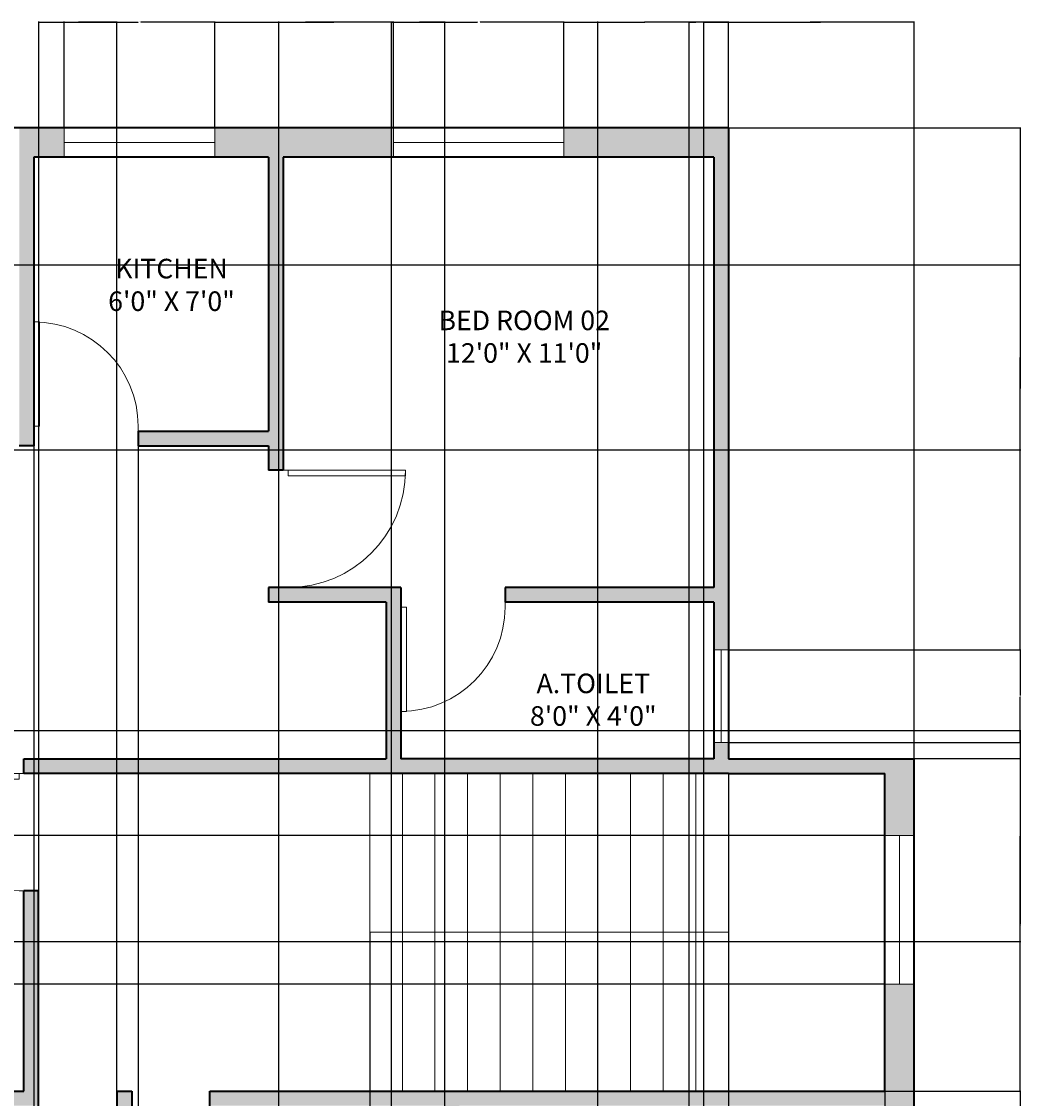
# Model space of a CAD drawing. Units: inches. Extents: x 2510 to 3056, y 673 to 1386.
# Tile 4 of 4: x 2749 to 3056, y 1056 to 1386. Entities that reach past the tile are written whole.
import ezdxf

# ---------------------------------------------------------------- set-up
doc = ezdxf.new("R2010")
doc.units = ezdxf.units.IN
for name, color, linetype, lineweight in [('A-ANNO-DIMS', 2, 'Continuous', 18), ('A-AREA-IDEN', 7, 'Continuous', 18), ('A-DOOR', 3, 'Continuous', 18), ('A-FLOR-STRS', 7, 'Continuous', 18), ('A-GLAZ', 4, 'Continuous', 18), ('A-WALL', 7, 'Continuous', 35), ('A-WALL-PATT', 252, 'Continuous', 13)]:
    doc.layers.add(name, color=color, linetype=linetype, lineweight=lineweight)
doc.styles.get("Standard").update_dxf_attribs({"font": 'arial.ttf'})
doc.dimstyles.get("Standard").update_dxf_attribs({"dimtxt": 0.18, "dimasz": 0.18, "dimexe": 0.18, "dimexo": 0.0625, "dimgap": 0.09, "dimtad": 0, "dimtih": 1, "dimtoh": 1, "dimdec": 4, "dimzin": 0, "dimdsep": 46, "dimtxsty": 'Standard', "dimcen": 0.09, "dimadec": 0, "dimazin": 0, "dimtfac": 1, "dimtdec": 4, "dimtofl": 0, "dimtmove": 0, "dimatfit": 3, "dimfxl": 1, "dimtolj": 1, "dimtzin": 0, "dimarcsym": 0})

# ---------------------------------------------------------------- blocks, each defined once
blk = doc.blocks.new('*U5')
for p, q in [((0, 0), (0, 6)), ((32, 0), (32, 6))]:
    blk.add_line(p, q)
blk.add_lwpolyline([(0, 0), (0, -32), (1.75, -32), (1.75, 0)], close=True)
blk.add_arc((0, 0), 32, 270, 0)
blk = doc.blocks.new('*U6')
for p, q in [((0, 0), (0, -6)), ((36, 0), (36, -6))]:
    blk.add_line(p, q)
blk.add_lwpolyline([(0, 0), (0, 36), (1.75, 36), (1.75, 0)], close=True)
blk.add_arc((0, 0), 36, 0, 90)
blk = doc.blocks.new('*U2')
for p, q in [((0, 0), (0, -6)), ((32, 0), (32, -6))]:
    blk.add_line(p, q)
blk.add_lwpolyline([(0, 0), (0, 32), (1.75, 32), (1.75, 0)], close=True)
blk.add_arc((0, 0), 32, 0, 90)
blk = doc.blocks.new('*U4')
for p, q in [((0, 0), (0, -6)), ((-36, 0), (-36, -6))]:
    blk.add_line(p, q)
blk.add_lwpolyline([(0, 0), (0, 36), (-1.75, 36), (-1.75, 0)], close=True)
blk.add_arc((0, 0), 36, 90, 180)
blk = doc.blocks.new('*U8')
for p, q in [((-24, 0), (-24, 6)), ((0, 0), (0, 6))]:
    blk.add_line(p, q)
blk.add_lwpolyline([(0, 0), (0, -24), (-1.75, -24), (-1.75, 0)], close=True)
blk.add_arc((0, 0), 24, 180, 270)
blk = doc.blocks.new('*U7')
for p, q in [((0, 0), (0, 6)), ((24, 0), (24, 6))]:
    blk.add_line(p, q)
blk.add_lwpolyline([(0, 0), (0, -24), (1.75, -24), (1.75, 0)], close=True)
blk.add_arc((0, 0), 24, 270, 0)
blk = doc.blocks.new('*D18')
at = {"layer": 'A-ANNO-DIMS', "color": 0, "lineweight": -2, "transparency": 16777216}
for p, q in [((2762.47, 1353.65), (2762.47, 1386.25)), ((2762.65, 1386.07), (2785.17, 1386.07)), ((2808.48, 1386.07), (2785.96, 1386.07)), ((2808.66, 1353.65), (2808.66, 1386.25))]:
    blk.add_line(p, q, dxfattribs=at)
at = {"layer": 'A-ANNO-DIMS', "color": 0, "transparency": 16777216}
for points in [[(2762.65, 1386.1), (2762.65, 1386.04), (2762.47, 1386.07)], [(2808.48, 1386.1), (2808.48, 1386.04), (2808.66, 1386.07)]]:
    blk.add_solid(points, dxfattribs=at)
at = {"layer": 'Defpoints', "color": 0, "transparency": 16777216}
for p in [(2808.66, 1386.07), (2762.47, 1353.59), (2808.66, 1353.59)]:
    blk.add_point(p, dxfattribs=at)
at = {"layer": 'A-ANNO-DIMS', "color": 0, "transparency": 16777216, "insert": (2785.57, 1386.07), "char_height": 0.18, "attachment_point": 5}
blk.add_mtext('\\A1;46.19', dxfattribs=at)
blk = doc.blocks.new('*D19')
at = {"layer": 'A-ANNO-DIMS', "color": 0, "lineweight": -2, "transparency": 16777216}
for p, q in [((2808.66, 1353.65), (2808.66, 1386.25)), ((2808.84, 1386.07), (2835.69, 1386.07)), ((2863.32, 1386.07), (2836.48, 1386.07)), ((2863.5, 1353.65), (2863.5, 1386.25))]:
    blk.add_line(p, q, dxfattribs=at)
at = {"layer": 'A-ANNO-DIMS', "color": 0, "transparency": 16777216}
for points in [[(2808.84, 1386.1), (2808.84, 1386.04), (2808.66, 1386.07)], [(2863.32, 1386.1), (2863.32, 1386.04), (2863.5, 1386.07)]]:
    blk.add_solid(points, dxfattribs=at)
at = {"layer": 'Defpoints', "color": 0, "transparency": 16777216}
for p in [(2863.5, 1386.07), (2808.66, 1353.59), (2863.5, 1353.59)]:
    blk.add_point(p, dxfattribs=at)
at = {"layer": 'A-ANNO-DIMS', "color": 0, "transparency": 16777216, "insert": (2836.08, 1386.07), "char_height": 0.18, "attachment_point": 5}
blk.add_mtext('\\A1;54.84', dxfattribs=at)
blk = doc.blocks.new('*D20')
at = {"layer": 'A-ANNO-DIMS', "color": 0, "lineweight": -2, "transparency": 16777216}
for p, q in [((2863.5, 1353.65), (2863.5, 1386.25)), ((2863.68, 1386.07), (2889.22, 1386.07)), ((2915.55, 1386.07), (2890.01, 1386.07)), ((2915.73, 1353.65), (2915.73, 1386.25))]:
    blk.add_line(p, q, dxfattribs=at)
at = {"layer": 'A-ANNO-DIMS', "color": 0, "transparency": 16777216}
for points in [[(2863.68, 1386.1), (2863.68, 1386.04), (2863.5, 1386.07)], [(2915.55, 1386.1), (2915.55, 1386.04), (2915.73, 1386.07)]]:
    blk.add_solid(points, dxfattribs=at)
at = {"layer": 'Defpoints', "color": 0, "transparency": 16777216}
for p in [(2915.73, 1386.07), (2863.5, 1353.59), (2915.73, 1353.59)]:
    blk.add_point(p, dxfattribs=at)
at = {"layer": 'A-ANNO-DIMS', "color": 0, "transparency": 16777216, "insert": (2889.61, 1386.07), "char_height": 0.18, "attachment_point": 5}
blk.add_mtext('\\A1;52.23', dxfattribs=at)
blk = doc.blocks.new('*D21')
at = {"layer": 'A-ANNO-DIMS', "color": 0, "lineweight": -2, "transparency": 16777216}
for p, q in [((2966.19, 1160.15), (2966.19, 1386.25)), ((2966.37, 1386.07), (2994.47, 1386.07)), ((3023.01, 1386.07), (2994.91, 1386.07)), ((3023.19, 1160.15), (3023.19, 1386.25))]:
    blk.add_line(p, q, dxfattribs=at)
at = {"layer": 'A-ANNO-DIMS', "color": 0, "transparency": 16777216}
for points in [[(2966.37, 1386.1), (2966.37, 1386.04), (2966.19, 1386.07)], [(3023.01, 1386.1), (3023.01, 1386.04), (3023.19, 1386.07)]]:
    blk.add_solid(points, dxfattribs=at)
at = {"layer": 'Defpoints', "color": 0, "transparency": 16777216}
for p in [(3023.19, 1386.07), (2966.19, 1160.09), (3023.19, 1160.09)]:
    blk.add_point(p, dxfattribs=at)
at = {"layer": 'A-ANNO-DIMS', "color": 0, "transparency": 16777216, "insert": (2994.69, 1386.07), "char_height": 0.18, "attachment_point": 5}
blk.add_mtext('\\A1;57', dxfattribs=at)
blk = doc.blocks.new('*D28')
at = {"layer": 'A-ANNO-DIMS', "color": 0, "lineweight": -2, "transparency": 16777216}
for p, q in [((3014.25, 1058.09), (3055.85, 1058.09)), ((3055.67, 1057.91), (3055.67, 1043.24)), ((3055.67, 1028.21), (3055.67, 1042.88)), ((3023.25, 1028.03), (3055.85, 1028.03))]:
    blk.add_line(p, q, dxfattribs=at)
at = {"layer": 'A-ANNO-DIMS', "color": 0, "transparency": 16777216}
for points in [[(3055.64, 1057.91), (3055.7, 1057.91), (3055.67, 1058.09)], [(3055.64, 1028.21), (3055.7, 1028.21), (3055.67, 1028.03)]]:
    blk.add_solid(points, dxfattribs=at)
at = {"layer": 'Defpoints', "color": 0, "transparency": 16777216}
for p in [(3014.19, 1058.09), (3055.67, 1058.09), (3023.19, 1028.03)]:
    blk.add_point(p, dxfattribs=at)
at = {"layer": 'A-ANNO-DIMS', "color": 0, "transparency": 16777216, "insert": (3055.67, 1043.06), "char_height": 0.18, "attachment_point": 5}
blk.add_mtext('\\A1;30.053', dxfattribs=at)
blk = doc.blocks.new('*D29')
at = {"layer": 'A-ANNO-DIMS', "color": 0, "lineweight": -2, "transparency": 16777216}
for p, q in [((3023.25, 1160.09), (3055.85, 1160.09)), ((3055.67, 1159.91), (3055.67, 1109.27)), ((3055.67, 1058.27), (3055.67, 1108.9)), ((3014.25, 1058.09), (3055.85, 1058.09))]:
    blk.add_line(p, q, dxfattribs=at)
at = {"layer": 'A-ANNO-DIMS', "color": 0, "transparency": 16777216}
for points in [[(3055.64, 1159.91), (3055.7, 1159.91), (3055.67, 1160.09)], [(3055.64, 1058.27), (3055.7, 1058.27), (3055.67, 1058.09)]]:
    blk.add_solid(points, dxfattribs=at)
at = {"layer": 'Defpoints', "color": 0, "transparency": 16777216}
for p in [(3023.19, 1160.09), (3055.67, 1160.09), (3014.19, 1058.09)]:
    blk.add_point(p, dxfattribs=at)
at = {"layer": 'A-ANNO-DIMS', "color": 0, "transparency": 16777216, "insert": (3055.67, 1109.09), "char_height": 0.18, "attachment_point": 5}
blk.add_mtext('\\A1;102', dxfattribs=at)
blk = doc.blocks.new('*D30')
at = {"layer": 'A-ANNO-DIMS', "color": 0, "lineweight": -2, "transparency": 16777216}
for p, q in [((2966.25, 1193.43), (3055.85, 1193.43)), ((3055.67, 1193.25), (3055.67, 1179.42)), ((3055.67, 1165.21), (3055.67, 1179.05)), ((2966.25, 1165.03), (3055.85, 1165.03))]:
    blk.add_line(p, q, dxfattribs=at)
at = {"layer": 'A-ANNO-DIMS', "color": 0, "transparency": 16777216}
for points in [[(3055.64, 1193.25), (3055.7, 1193.25), (3055.67, 1193.43)], [(3055.64, 1165.21), (3055.7, 1165.21), (3055.67, 1165.03)]]:
    blk.add_solid(points, dxfattribs=at)
at = {"layer": 'Defpoints', "color": 0, "transparency": 16777216}
for p in [(2966.19, 1193.43), (3055.67, 1193.43), (2966.19, 1165.03)]:
    blk.add_point(p, dxfattribs=at)
at = {"layer": 'A-ANNO-DIMS', "color": 0, "transparency": 16777216, "insert": (3055.67, 1179.23), "char_height": 0.18, "attachment_point": 5}
blk.add_mtext('\\A1;28.4', dxfattribs=at)
blk = doc.blocks.new('*D31')
at = {"layer": 'A-ANNO-DIMS', "color": 0, "lineweight": -2, "transparency": 16777216}
for p, q in [((2966.25, 1353.59), (3055.85, 1353.59)), ((3055.67, 1353.41), (3055.67, 1273.69)), ((3055.67, 1193.61), (3055.67, 1273.33)), ((2966.25, 1193.43), (3055.85, 1193.43))]:
    blk.add_line(p, q, dxfattribs=at)
at = {"layer": 'A-ANNO-DIMS', "color": 0, "transparency": 16777216}
for points in [[(3055.64, 1353.41), (3055.7, 1353.41), (3055.67, 1353.59)], [(3055.64, 1193.61), (3055.7, 1193.61), (3055.67, 1193.43)]]:
    blk.add_solid(points, dxfattribs=at)
at = {"layer": 'Defpoints', "color": 0, "transparency": 16777216}
for p in [(2966.19, 1353.59), (3055.67, 1353.59), (2966.19, 1193.43)]:
    blk.add_point(p, dxfattribs=at)
at = {"layer": 'A-ANNO-DIMS', "color": 0, "transparency": 16777216, "insert": (3055.67, 1273.51), "char_height": 0.18, "attachment_point": 5}
blk.add_mtext('\\A1;160.15', dxfattribs=at)
blk = doc.blocks.new('*D32')
at = {"layer": 'A-ANNO-DIMS', "color": 0, "lineweight": -2, "transparency": 16777216}
for p, q in [((3014.13, 1136.48), (2510.53, 1136.48)), ((2510.71, 1136.3), (2510.71, 1113.86)), ((2510.71, 1091.06), (2510.71, 1113.5)), ((3014.13, 1090.88), (2510.53, 1090.88))]:
    blk.add_line(p, q, dxfattribs=at)
at = {"layer": 'A-ANNO-DIMS', "color": 0, "transparency": 16777216}
for points in [[(2510.68, 1136.3), (2510.74, 1136.3), (2510.71, 1136.48)], [(2510.68, 1091.06), (2510.74, 1091.06), (2510.71, 1090.88)]]:
    blk.add_solid(points, dxfattribs=at)
at = {"layer": 'Defpoints', "color": 0, "transparency": 16777216}
for p in [(2510.71, 1136.48), (3014.19, 1136.48), (3014.19, 1090.88)]:
    blk.add_point(p, dxfattribs=at)
at = {"layer": 'A-ANNO-DIMS', "color": 0, "transparency": 16777216, "insert": (2510.71, 1113.68), "char_height": 0.18, "attachment_point": 5}
blk.add_mtext('\\A1;45.6', dxfattribs=at)
blk = doc.blocks.new('*D36')
at = {"layer": 'A-ANNO-DIMS', "color": 0, "lineweight": -2, "transparency": 16777216}
for p, q in [((2552.25, 1168.75), (3055.85, 1168.75)), ((3055.67, 1168.57), (3055.67, 1136.56)), ((3055.67, 1104.19), (3055.67, 1136.2)), ((2552.25, 1104.01), (3055.85, 1104.01))]:
    blk.add_line(p, q, dxfattribs=at)
at = {"layer": 'A-ANNO-DIMS', "color": 0, "transparency": 16777216}
for points in [[(3055.64, 1168.57), (3055.7, 1168.57), (3055.67, 1168.75)], [(3055.64, 1104.19), (3055.7, 1104.19), (3055.67, 1104.01)]]:
    blk.add_solid(points, dxfattribs=at)
at = {"layer": 'Defpoints', "color": 0, "transparency": 16777216}
for p in [(2552.19, 1168.75), (3055.67, 1168.75), (2552.19, 1104.01)]:
    blk.add_point(p, dxfattribs=at)
at = {"layer": 'A-ANNO-DIMS', "color": 0, "transparency": 16777216, "insert": (3055.67, 1136.38), "char_height": 0.18, "attachment_point": 5}
blk.add_mtext('\\A1;64.74', dxfattribs=at)
blk = doc.blocks.new('*D37')
at = {"layer": 'A-ANNO-DIMS', "color": 0, "lineweight": -2, "transparency": 16777216}
for p, q in [((2552.25, 1311.56), (3055.85, 1311.56)), ((3055.67, 1311.38), (3055.67, 1283.38)), ((3055.67, 1255.02), (3055.67, 1283.02)), ((2552.25, 1254.84), (3055.85, 1254.84))]:
    blk.add_line(p, q, dxfattribs=at)
at = {"layer": 'A-ANNO-DIMS', "color": 0, "transparency": 16777216}
for points in [[(3055.64, 1311.38), (3055.7, 1311.38), (3055.67, 1311.56)], [(3055.64, 1255.02), (3055.7, 1255.02), (3055.67, 1254.84)]]:
    blk.add_solid(points, dxfattribs=at)
at = {"layer": 'Defpoints', "color": 0, "transparency": 16777216}
for p in [(2552.19, 1311.56), (3055.67, 1311.56), (2552.19, 1254.84)]:
    blk.add_point(p, dxfattribs=at)
at = {"layer": 'A-ANNO-DIMS', "color": 0, "transparency": 16777216, "insert": (3055.67, 1283.2), "char_height": 0.18, "attachment_point": 5}
blk.add_mtext('\\A1;56.72', dxfattribs=at)
blk = doc.blocks.new('*D38')
at = {"layer": 'A-ANNO-DIMS', "color": 0, "lineweight": -2, "transparency": 16777216}
for p, q in [((2856.19, 1106.77), (2856.19, 672.93)), ((2966.19, 1106.77), (2966.19, 672.93)), ((2856.37, 673.11), (2910.91, 673.11)), ((2966.01, 673.11), (2911.47, 673.11))]:
    blk.add_line(p, q, dxfattribs=at)
at = {"layer": 'A-ANNO-DIMS', "color": 0, "transparency": 16777216}
for points in [[(2856.37, 673.14), (2856.37, 673.08), (2856.19, 673.11)], [(2966.01, 673.14), (2966.01, 673.08), (2966.19, 673.11)]]:
    blk.add_solid(points, dxfattribs=at)
at = {"layer": 'Defpoints', "color": 0, "transparency": 16777216}
for p in [(2856.19, 1106.84), (2966.19, 1106.84), (2966.19, 673.11)]:
    blk.add_point(p, dxfattribs=at)
at = {"layer": 'A-ANNO-DIMS', "color": 0, "transparency": 16777216, "insert": (2911.19, 673.11), "char_height": 0.18, "attachment_point": 5}
blk.add_mtext('\\A1;110', dxfattribs=at)
blk = doc.blocks.new('*D39')
at = {"layer": 'A-ANNO-DIMS', "color": 0, "lineweight": -2, "transparency": 16777216}
for p, q in [((2966.19, 1155.52), (2966.19, 672.93)), ((3014.19, 1155.52), (3014.19, 672.93)), ((2966.37, 673.11), (2989.97, 673.11)), ((3014.01, 673.11), (2990.42, 673.11))]:
    blk.add_line(p, q, dxfattribs=at)
at = {"layer": 'A-ANNO-DIMS', "color": 0, "transparency": 16777216}
for points in [[(2966.37, 673.14), (2966.37, 673.08), (2966.19, 673.11)], [(3014.01, 673.14), (3014.01, 673.08), (3014.19, 673.11)]]:
    blk.add_solid(points, dxfattribs=at)
at = {"layer": 'Defpoints', "color": 0, "transparency": 16777216}
for p in [(2966.19, 1155.59), (3014.19, 1155.59), (3014.19, 673.11)]:
    blk.add_point(p, dxfattribs=at)
at = {"layer": 'A-ANNO-DIMS', "color": 0, "transparency": 16777216, "insert": (2990.19, 673.11), "char_height": 0.18, "attachment_point": 5}
blk.add_mtext('\\A1;48', dxfattribs=at)
blk = doc.blocks.new('*D42')
at = {"layer": 'A-ANNO-DIMS', "color": 0, "lineweight": -2, "transparency": 16777216}
for p, q in [((2828.31, 719.15), (2828.31, 1386.25)), ((2828.49, 1386.07), (2845.18, 1386.07)), ((2862.66, 1386.07), (2845.97, 1386.07)), ((2862.84, 719.15), (2862.84, 1386.25))]:
    blk.add_line(p, q, dxfattribs=at)
at = {"layer": 'A-ANNO-DIMS', "color": 0, "transparency": 16777216}
for points in [[(2828.49, 1386.1), (2828.49, 1386.04), (2828.31, 1386.07)], [(2862.66, 1386.1), (2862.66, 1386.04), (2862.84, 1386.07)]]:
    blk.add_solid(points, dxfattribs=at)
at = {"layer": 'Defpoints', "color": 0, "transparency": 16777216}
for p in [(2862.84, 1386.07), (2828.31, 719.09), (2862.84, 719.09)]:
    blk.add_point(p, dxfattribs=at)
at = {"layer": 'A-ANNO-DIMS', "color": 0, "transparency": 16777216, "insert": (2845.57, 1386.07), "char_height": 0.18, "attachment_point": 5}
blk.add_mtext('\\A1;34.53', dxfattribs=at)
blk = doc.blocks.new('*D43')
at = {"layer": 'A-ANNO-DIMS', "color": 0, "lineweight": -2, "transparency": 16777216}
for p, q in [((2862.84, 719.15), (2862.84, 1386.25)), ((2863.02, 1386.07), (2870.56, 1386.07)), ((2879.01, 1386.07), (2871.47, 1386.07)), ((2879.19, 719.15), (2879.19, 1386.25))]:
    blk.add_line(p, q, dxfattribs=at)
at = {"layer": 'A-ANNO-DIMS', "color": 0, "transparency": 16777216}
for points in [[(2863.02, 1386.1), (2863.02, 1386.04), (2862.84, 1386.07)], [(2879.01, 1386.1), (2879.01, 1386.04), (2879.19, 1386.07)]]:
    blk.add_solid(points, dxfattribs=at)
at = {"layer": 'Defpoints', "color": 0, "transparency": 16777216}
for p in [(2879.19, 1386.07), (2862.84, 719.09), (2879.19, 719.09)]:
    blk.add_point(p, dxfattribs=at)
at = {"layer": 'A-ANNO-DIMS', "color": 0, "transparency": 16777216, "insert": (2871.02, 1386.07), "char_height": 0.18, "attachment_point": 5}
blk.add_mtext('\\A1;16.354', dxfattribs=at)
blk = doc.blocks.new('*D44')
at = {"layer": 'A-ANNO-DIMS', "color": 0, "lineweight": -2, "transparency": 16777216}
for p, q in [((2754.69, 1058.15), (2754.69, 1386.25)), ((2754.87, 1386.07), (2766.47, 1386.07)), ((2778.51, 1386.07), (2766.91, 1386.07)), ((2778.69, 1058.15), (2778.69, 1386.25))]:
    blk.add_line(p, q, dxfattribs=at)
at = {"layer": 'A-ANNO-DIMS', "color": 0, "transparency": 16777216}
for points in [[(2754.87, 1386.1), (2754.87, 1386.04), (2754.69, 1386.07)], [(2778.51, 1386.1), (2778.51, 1386.04), (2778.69, 1386.07)]]:
    blk.add_solid(points, dxfattribs=at)
at = {"layer": 'Defpoints', "color": 0, "transparency": 16777216}
for p in [(2778.69, 1386.07), (2754.69, 1058.09), (2778.69, 1058.09)]:
    blk.add_point(p, dxfattribs=at)
at = {"layer": 'A-ANNO-DIMS', "color": 0, "transparency": 16777216, "insert": (2766.69, 1386.07), "char_height": 0.18, "attachment_point": 5}
blk.add_mtext('\\A1;24', dxfattribs=at)
blk = doc.blocks.new('*D46')
at = {"layer": 'A-ANNO-DIMS', "color": 0, "lineweight": -2, "transparency": 16777216}
for p, q in [((2753.19, 1256.02), (2753.19, 672.93)), ((2785.19, 1256.02), (2785.19, 672.93)), ((2753.37, 673.11), (2768.97, 673.11)), ((2785.01, 673.11), (2769.41, 673.11))]:
    blk.add_line(p, q, dxfattribs=at)
at = {"layer": 'A-ANNO-DIMS', "color": 0, "transparency": 16777216}
for points in [[(2753.37, 673.14), (2753.37, 673.08), (2753.19, 673.11)], [(2785.01, 673.14), (2785.01, 673.08), (2785.19, 673.11)]]:
    blk.add_solid(points, dxfattribs=at)
at = {"layer": 'Defpoints', "color": 0, "transparency": 16777216}
for p in [(2753.19, 1256.09), (2785.19, 1256.09), (2785.19, 673.11)]:
    blk.add_point(p, dxfattribs=at)
at = {"layer": 'A-ANNO-DIMS', "color": 0, "transparency": 16777216, "insert": (2769.19, 673.11), "char_height": 0.18, "attachment_point": 5}
blk.add_mtext('\\A1;32', dxfattribs=at)
blk = doc.blocks.new('*D47')
at = {"layer": 'A-ANNO-DIMS', "color": 0, "lineweight": -2, "transparency": 16777216}
for p, q in [((2926.19, 750.65), (2926.19, 1386.25)), ((2926.37, 1386.07), (2939.97, 1386.07)), ((2954.01, 1386.07), (2940.41, 1386.07)), ((2954.19, 750.65), (2954.19, 1386.25))]:
    blk.add_line(p, q, dxfattribs=at)
at = {"layer": 'A-ANNO-DIMS', "color": 0, "transparency": 16777216}
for points in [[(2926.37, 1386.1), (2926.37, 1386.04), (2926.19, 1386.07)], [(2954.01, 1386.1), (2954.01, 1386.04), (2954.19, 1386.07)]]:
    blk.add_solid(points, dxfattribs=at)
at = {"layer": 'Defpoints', "color": 0, "transparency": 16777216}
for p in [(2954.19, 1386.07), (2926.19, 750.59), (2954.19, 750.59)]:
    blk.add_point(p, dxfattribs=at)
at = {"layer": 'A-ANNO-DIMS', "color": 0, "transparency": 16777216, "insert": (2940.19, 1386.07), "char_height": 0.18, "attachment_point": 5}
blk.add_mtext('\\A1;28', dxfattribs=at)
blk = doc.blocks.new('*D56')
at = {"layer": 'A-ANNO-DIMS', "color": 0, "lineweight": -2, "transparency": 16777216}
for p, q in [((2954.19, 750.65), (2954.19, 1386.25)), ((2954.37, 1386.07), (2956.18, 1386.07)), ((2958.51, 1386.07), (2956.7, 1386.07)), ((2958.69, 750.65), (2958.69, 1386.25))]:
    blk.add_line(p, q, dxfattribs=at)
at = {"layer": 'A-ANNO-DIMS', "color": 0, "transparency": 16777216}
for points in [[(2954.37, 1386.1), (2954.37, 1386.04), (2954.19, 1386.07)], [(2958.51, 1386.1), (2958.51, 1386.04), (2958.69, 1386.07)]]:
    blk.add_solid(points, dxfattribs=at)
at = {"layer": 'Defpoints', "color": 0, "transparency": 16777216}
for p in [(2958.69, 1386.07), (2954.19, 750.59), (2958.69, 750.59)]:
    blk.add_point(p, dxfattribs=at)
at = {"layer": 'A-ANNO-DIMS', "color": 0, "transparency": 16777216, "insert": (2956.44, 1386.07), "char_height": 0.18, "attachment_point": 5}
blk.add_mtext('\\A1;4.5', dxfattribs=at)
blk = doc.blocks.new('*D58')
at = {"layer": 'A-ANNO-DIMS', "color": 0, "lineweight": -2, "transparency": 16777216}
for p, q in [((2958.69, 705.65), (2958.69, 1386.25)), ((2958.87, 1386.07), (2990.62, 1386.07)), ((3023.01, 1386.07), (2991.27, 1386.07)), ((3023.19, 705.65), (3023.19, 1386.25))]:
    blk.add_line(p, q, dxfattribs=at)
at = {"layer": 'A-ANNO-DIMS', "color": 0, "transparency": 16777216}
for points in [[(2958.87, 1386.1), (2958.87, 1386.04), (2958.69, 1386.07)], [(3023.01, 1386.1), (3023.01, 1386.04), (3023.19, 1386.07)]]:
    blk.add_solid(points, dxfattribs=at)
at = {"layer": 'Defpoints', "color": 0, "transparency": 16777216}
for p in [(3023.19, 1386.07), (2958.69, 705.59), (3023.19, 705.59)]:
    blk.add_point(p, dxfattribs=at)
at = {"layer": 'A-ANNO-DIMS', "color": 0, "transparency": 16777216, "insert": (2990.94, 1386.07), "char_height": 0.18, "attachment_point": 5}
blk.add_mtext('\\A1;64.5', dxfattribs=at)
blk = doc.blocks.new('*D59')
at = {"layer": 'A-ANNO-DIMS', "color": 0, "lineweight": -2, "transparency": 16777216}
for p, q in [((2915.73, 1353.65), (2915.73, 1386.25)), ((2915.91, 1386.07), (2940.57, 1386.07)), ((2966.01, 1386.07), (2941.35, 1386.07)), ((2966.19, 1353.65), (2966.19, 1386.25))]:
    blk.add_line(p, q, dxfattribs=at)
at = {"layer": 'A-ANNO-DIMS', "color": 0, "transparency": 16777216}
for points in [[(2915.91, 1386.1), (2915.91, 1386.04), (2915.73, 1386.07)], [(2966.01, 1386.1), (2966.01, 1386.04), (2966.19, 1386.07)]]:
    blk.add_solid(points, dxfattribs=at)
at = {"layer": 'Defpoints', "color": 0, "transparency": 16777216}
for p in [(2966.19, 1386.07), (2915.73, 1353.59), (2966.19, 1353.59)]:
    blk.add_point(p, dxfattribs=at)
at = {"layer": 'A-ANNO-DIMS', "color": 0, "transparency": 16777216, "insert": (2940.96, 1386.07), "char_height": 0.18, "attachment_point": 5}
blk.add_mtext('\\A1;50.46', dxfattribs=at)

msp = doc.modelspace()

# ---------------------------------------------------------------- hatches: boundary and pattern name
at = {"layer": 'A-WALL-PATT'}
h = msp.add_hatch(color=256, dxfattribs=at)
h.dxf.hatch_style = 1
h.paths.add_polyline_path([(2580.5162, 1353.5862), (2543.1924, 1353.5862), (2543.1924, 1311.5591), (2552.1924, 1311.5591), (2552.1924, 1344.5862), (2580.5162, 1344.5862)])
h.paths.add_polyline_path([(2720.7125, 1353.5862), (2648.0497, 1353.5862), (2648.0497, 1344.5862), (2696.1924, 1344.5862), (2696.1924, 1208.0862), (2700.6924, 1208.0862), (2700.6924, 1256.0862), (2716.6924, 1256.0862), (2716.6924, 1260.5862), (2700.6924, 1260.5862), (2700.6924, 1344.5862), (2720.7125, 1344.5862)])
h.paths.add_polyline_path([(2762.4727, 1353.5862), (2748.6924, 1353.5862), (2748.6924, 1344.5862), (2748.6924, 1256.0862), (2753.1924, 1256.0862), (2753.1924, 1262.0862), (2753.1924, 1294.0862), (2753.1924, 1344.5862), (2762.4727, 1344.5862)])
h.paths.add_polyline_path([(2863.5016, 1353.5862), (2808.6621, 1353.5862), (2808.6621, 1344.5862), (2825.1924, 1344.5862), (2825.1924, 1260.5862), (2785.1924, 1260.5862), (2785.1924, 1256.0862), (2825.1924, 1256.0862), (2825.1924, 1248.5862), (2829.6924, 1248.5862), (2829.6924, 1344.5862), (2863.5016, 1344.5862)])
h.paths.add_polyline_path([(2966.1924, 1353.5862), (2915.7284, 1353.5862), (2915.7284, 1344.5862), (2961.6924, 1344.5862), (2961.6924, 1212.5862), (2897.6924, 1212.5862), (2897.6924, 1208.0862), (2961.6924, 1208.0862), (2961.6924, 1193.4346), (2966.1924, 1193.4346), (2966.1924, 1208.0862)])
h.paths.add_polyline_path([(2660.1924, 1212.5862), (2552.1924, 1212.5862), (2552.1924, 1254.8401), (2543.1924, 1254.8401), (2543.1924, 1168.7504), (2552.1924, 1168.7504), (2552.1924, 1208.0862), (2660.1924, 1208.0862)])
h.paths.add_polyline_path([(3023.1924, 1160.0862), (2966.1924, 1160.0862), (2966.1924, 1165.033), (2961.6924, 1165.033), (2961.6924, 1160.0862), (2865.6924, 1160.0862), (2865.6924, 1212.5862), (2825.1924, 1212.5862), (2825.1924, 1208.0862), (2861.1924, 1208.0862), (2861.1924, 1160.0862), (2750.1527, 1160.0862), (2750.1527, 1155.5862), (2754.6527, 1155.5862), (2966.1924, 1155.5862), (3014.1924, 1155.5862), (3014.1924, 1136.4806), (3023.1924, 1136.4806)])
h.paths.add_polyline_path([(3023.1924, 1090.8839), (3014.1924, 1090.8839), (3014.1924, 1058.0862), (2807.1924, 1058.0862), (2807.1924, 1053.5862), (2879.1924, 1053.5862), (2879.1924, 929.0862), (2883.6924, 929.0862), (2883.6924, 935.0862), (2883.6924, 971.0862), (2883.6924, 1053.5862), (3014.1924, 1053.5862), (3014.1924, 1028.0329), (3023.1924, 1028.0329)])
h.paths.add_polyline_path([(3023.1924, 970.6943), (3014.1924, 970.6943), (3014.1924, 933.5862), (2919.6924, 933.5862), (2919.6924, 929.0862), (2927.1924, 929.0862), (2927.1924, 907.0862), (2931.6924, 907.0862), (2931.6924, 929.0862), (3014.1924, 929.0862), (3014.1924, 918.5377), (3023.1924, 918.5377)])
h.paths.add_polyline_path([(3023.1924, 886.219), (3014.1924, 886.219), (3014.1924, 875.0862), (2927.1924, 875.0862), (2879.1924, 875.0862), (2879.1924, 870.5862), (2885.1924, 870.5862), (2921.1924, 870.5862), (3014.1924, 870.5862), (3014.1924, 835.4806), (3023.1924, 835.4806)])
h.paths.add_polyline_path([(3023.1924, 775.6299), (3014.1924, 775.6299), (3014.1924, 746.0862), (3023.1924, 746.0862)])
h.paths.add_polyline_path([(2958.6924, 750.5862), (2954.1924, 750.5862), (2954.1924, 744.5862), (2954.1924, 716.5862), (2954.1924, 710.0862), (2910.6841, 710.0862), (2910.6841, 705.5862), (2958.6924, 705.5862)])
h.paths.add_polyline_path([(2926.1924, 750.5862), (2883.6924, 750.5862), (2883.6924, 834.5862), (2879.1924, 834.5862), (2879.1924, 819.5862), (2815.1924, 819.5862), (2815.1924, 815.0862), (2879.1924, 815.0862), (2879.1924, 746.0862), (2879.1924, 719.0862), (2862.8388, 719.0862), (2862.8388, 714.5862), (2879.1924, 714.5862), (2879.1924, 705.5862), (2883.6924, 705.5862), (2883.6924, 710.0862), (2883.6924, 746.0862), (2926.1924, 746.1758)])
h.paths.add_polyline_path([(2682.6924, 815.0862), (2746.6924, 815.0862), (2746.6924, 819.5862), (2682.6924, 819.5862), (2682.6924, 834.5862), (2678.1924, 834.5862), (2678.1924, 750.5862), (2639.6924, 750.5862), (2639.6924, 746.0862), (2678.1924, 746.0862), (2678.1924, 710.0862), (2678.1924, 705.5862), (2682.6924, 705.5862), (2682.6924, 714.5862), (2699.7376, 714.5862), (2699.7376, 719.0862), (2682.6924, 719.0862), (2682.6924, 746.0862)])
h.paths.add_polyline_path([(2650.2761, 710.0862), (2607.6924, 710.0862), (2607.6924, 750.5862), (2603.1924, 750.5862), (2603.1924, 705.5862), (2607.6924, 705.5862), (2650.2761, 705.5862)])
h.paths.add_polyline_path([(2552.1924, 777.7158), (2543.1924, 777.7158), (2543.1924, 746.0862), (2552.1924, 746.0862)])
h.paths.add_polyline_path([(2828.3093, 719.0862), (2783.1924, 719.0862), (2783.1924, 815.0862), (2783.1924, 1058.0862), (2778.6924, 1058.0862), (2778.6924, 815.0862), (2778.6924, 719.0862), (2743.8813, 719.0862), (2743.8813, 714.5862), (2778.6924, 714.5862), (2828.3093, 714.5862)])
h.paths.add_polyline_path([(2642.1924, 933.5862), (2552.1924, 933.5862), (2552.1924, 965.3494), (2543.1924, 965.3494), (2543.1924, 907.809), (2552.1924, 907.809), (2552.1924, 929.0862), (2630.1924, 929.0862), (2630.1924, 907.0862), (2634.6924, 907.0862), (2634.6924, 929.0862), (2642.1924, 929.0862)])
h.paths.add_polyline_path([(2682.6924, 875.0862), (2552.1924, 875.0862), (2543.1924, 875.0862), (2543.1924, 832.3664), (2552.1924, 832.3664), (2552.1924, 870.5862), (2634.6924, 870.5862), (2682.6924, 870.5862)])
h.paths.add_polyline_path([(2754.6527, 1119.5862), (2750.1527, 1119.5862), (2750.1527, 1058.0862), (2552.1924, 1058.0862), (2552.1924, 1104.0128), (2543.1924, 1104.0128), (2543.1924, 1017.3235), (2552.1924, 1017.3235), (2552.1924, 1053.5862), (2678.1924, 1053.5862), (2678.1924, 929.0862), (2682.6924, 929.0862), (2682.6924, 1053.5862), (2754.6527, 1053.5862)])

# ---------------------------------------------------------------- linework, layer by layer
at = {"layer": 'A-FLOR-STRS'}
for p, q in [((2856.1924, 1155.5862), (2856.1924, 1058.0862)), ((2866.1924, 1155.5862), (2866.1924, 1058.0862)), ((2876.1924, 1155.5862), (2876.1924, 1058.0862)), ((2886.1924, 1155.5862), (2886.1924, 1058.0862)), ((2896.1924, 1155.5862), (2896.1924, 1058.0862)), ((2906.1924, 1155.5862), (2906.1924, 1058.0862)), ((2916.1924, 1155.5862), (2916.1924, 1058.0862)), ((2926.1924, 1155.5862), (2926.1924, 1058.0862)), ((2936.1924, 1155.5862), (2936.1924, 1058.0862)), ((2946.1924, 1155.5862), (2946.1924, 1058.0862)), ((2956.1924, 1155.5862), (2956.1924, 1058.0862)), ((2966.1924, 1155.5862), (2966.1924, 1058.0862)), ((2966.1924, 1106.8362), (2856.1924, 1106.8362))]:
    msp.add_line(p, q, dxfattribs=at)
at = {"layer": 'A-GLAZ'}
for p, q in [((2762.4727, 1344.5862), (2762.4727, 1353.5862)), ((2808.6621, 1344.5862), (2808.6621, 1353.5862)), ((2863.5016, 1344.5862), (2863.5016, 1353.5862)), ((2915.7284, 1353.5862), (2915.7284, 1344.5862)), ((2762.4727, 1349.0862), (2808.6621, 1349.0862)), ((2863.5016, 1349.0862), (2915.7284, 1349.0862)), ((2961.6924, 1193.4346), (2966.1924, 1193.4346)), ((2963.9424, 1165.033), (2963.9424, 1193.4346)), ((2961.6924, 1165.033), (2966.1924, 1165.033)), ((3014.1924, 1136.4806), (3023.1924, 1136.4806)), ((3018.6924, 1090.8839), (3018.6924, 1136.4806)), ((3014.1924, 1090.8839), (3023.1924, 1090.8839))]:
    msp.add_line(p, q, dxfattribs=at)
at = {"layer": 'A-WALL'}
for p, q in [((2966.1924, 1353.5862), (2543.1924, 1353.5862)), ((2966.1924, 1353.5862), (2966.1924, 1208.0862)), ((2753.1924, 1344.5862), (2753.1924, 1256.0862)), ((2825.1924, 1344.5862), (2753.1924, 1344.5862)), ((2825.1924, 1344.5862), (2825.1924, 1260.5862)), ((2961.6924, 1344.5862), (2829.6924, 1344.5862)), ((2829.6924, 1344.5862), (2829.6924, 1248.5862)), ((2961.6924, 1344.5862), (2961.6924, 1212.5862)), ((2785.1924, 1260.5862), (2785.1924, 1256.0862)), ((2785.1924, 1260.5862), (2825.1924, 1260.5862)), ((2753.1924, 1256.0862), (2748.6924, 1256.0862)), ((2785.1924, 1256.0862), (2825.1924, 1256.0862)), ((2825.1924, 1256.0862), (2825.1924, 1248.5862)), ((2829.6924, 1248.5862), (2825.1924, 1248.5862)), ((2825.1924, 1212.5862), (2825.1924, 1208.0862)), ((2865.6924, 1212.5862), (2825.1924, 1212.5862)), ((2865.6924, 1212.5862), (2865.6924, 1160.0862)), ((2961.6924, 1212.5862), (2897.6924, 1212.5862)), ((2897.6924, 1212.5862), (2897.6924, 1208.0862)), ((2861.1924, 1208.0862), (2825.1924, 1208.0862)), ((2861.1924, 1208.0862), (2861.1924, 1160.0862)), ((2961.6924, 1208.0862), (2897.6924, 1208.0862)), ((2961.6924, 1208.0862), (2961.6924, 1160.0862)), ((2966.1924, 1208.0862), (2966.1924, 1160.0862)), ((2750.1527, 1160.0862), (2861.1924, 1160.0862)), ((2750.1527, 1155.5862), (2750.1527, 1160.0862)), ((2961.6924, 1160.0862), (2865.6924, 1160.0862)), ((2966.1924, 1160.0862), (3023.1924, 1160.0862)), ((3023.1924, 705.5862), (3023.1924, 1160.0862)), ((2966.1924, 1155.5862), (2750.1527, 1155.5862)), ((2966.1924, 1155.5862), (3014.1924, 1155.5862)), ((3014.1924, 1058.0862), (3014.1924, 1155.5862)), ((2750.1527, 1058.0862), (2750.1527, 1119.5862)), ((2754.6527, 1119.5862), (2750.1527, 1119.5862)), ((2754.6527, 1053.5862), (2754.6527, 1119.5862)), ((2552.1924, 1058.0862), (2750.1527, 1058.0862)), ((2778.6924, 1058.0862), (2778.6924, 815.0862)), ((2778.6924, 1058.0862), (2783.1924, 1058.0862)), ((2783.1924, 1058.0862), (2783.1924, 815.0862)), ((2807.1924, 1053.5862), (2807.1924, 1058.0862)), ((2807.1924, 1058.0862), (3014.1924, 1058.0862))]:
    msp.add_line(p, q, dxfattribs=at)

# ---------------------------------------------------------------- block references
at = {"layer": 'A-DOOR'}
for name, p in [('*U2', (2753.1924, 1262.0862)), ('*U5', (2865.6924, 1206.5862)), ('*U8', (2778.6924, 1052.0862)), ('*U7', (2783.1924, 1052.0862))]:
    msp.add_blockref(name, p, dxfattribs=at)
for name, p, rotation in [('*U6', (2831.1924, 1248.5862), 270), ('*U4', (2748.6527, 1155.5862), 90)]:
    msp.add_blockref(name, p, dxfattribs=dict(at, rotation=rotation))

# ---------------------------------------------------------------- texts
at = {"layer": 'A-AREA-IDEN', "char_height": 6, "attachment_point": 1}
for s, insert in [('\\pxqc;KITCHEN\\P6\'0" X 7\'0"', (2765.6227, 1313.4501)), ('\\pxqc;BED ROOM 02\\P12\'0" X 11\'0"', (2873.7839, 1297.5557)), ('\\pxqc;A.TOILET\\P8\'0" X 4\'0"', (2894.9676, 1186.184))]:
    msp.add_mtext_dynamic_manual_height_columns(s, width=59.569763, gutter_width=12.5, heights=[0], dxfattribs=dict(at, insert=insert))

# ---------------------------------------------------------------- dimensions: what is measured, and where the dimension line sits
at = {"layer": 'A-ANNO-DIMS'}
for base, p1, p2, override, picture, middle in [((2778.6924, 1386.0667), (2754.6924, 1058.0862), (2778.6924, 1058.0862), {"dimdec": 0, "dimlfac": 1, "dimrnd": 0, "dimzin": 0, "dimdsep": 46, "dimlunit": 2}, '*D44', (2766.6924, 1386.0667)), ((2808.6621, 1386.0667), (2762.4727, 1353.5862), (2808.6621, 1353.5862), {"dimdec": 2, "dimlfac": 1, "dimrnd": 0, "dimzin": 0, "dimdsep": 46, "dimlunit": 2}, '*D18', (2785.5674, 1386.0667)), ((2863.5016, 1386.0667), (2808.6621, 1353.5862), (2863.5016, 1353.5862), {"dimdec": 2, "dimlfac": 1, "dimrnd": 0, "dimzin": 0, "dimdsep": 46, "dimlunit": 2}, '*D19', (2836.0818, 1386.0667)), ((2862.8388, 1386.0667), (2828.3093, 719.0862), (2862.8388, 719.0862), {"dimdec": 2, "dimlfac": 1, "dimrnd": 0, "dimzin": 0, "dimdsep": 46, "dimlunit": 2}, '*D42', (2845.5741, 1386.0667)), ((2879.1924, 1386.0667), (2862.8388, 719.0862), (2879.1924, 719.0862), {"dimdec": 3, "dimlfac": 1, "dimrnd": 0, "dimzin": 0, "dimdsep": 46, "dimlunit": 2}, '*D43', (2871.0156, 1386.0667)), ((2915.7284, 1386.0667), (2863.5016, 1353.5862), (2915.7284, 1353.5862), {"dimdec": 2, "dimlfac": 1, "dimrnd": 0, "dimzin": 0, "dimdsep": 46, "dimlunit": 2}, '*D20', (2889.615, 1386.0667)), ((2966.1924, 1386.0667), (2915.7284, 1353.5862), (2966.1924, 1353.5862), {"dimdec": 2, "dimlfac": 1, "dimrnd": 0, "dimzin": 0, "dimdsep": 46, "dimlunit": 2}, '*D59', (2940.9604, 1386.0667)), ((2954.1924, 1386.0667), (2926.1924, 750.5862), (2954.1924, 750.5862), {"dimdec": 0, "dimlfac": 1, "dimrnd": 0, "dimzin": 0, "dimdsep": 46, "dimlunit": 2}, '*D47', (2940.1924, 1386.0667)), ((2958.6924, 1386.0667), (2954.1924, 750.5862), (2958.6924, 750.5862), {"dimdec": 1, "dimlfac": 1, "dimrnd": 0, "dimzin": 0, "dimdsep": 46, "dimlunit": 2}, '*D56', (2956.4424, 1386.0667)), ((3023.1924, 1386.0667), (2958.6924, 705.5862), (3023.1924, 705.5862), {"dimdec": 1, "dimlfac": 1, "dimrnd": 0, "dimzin": 0, "dimdsep": 46, "dimlunit": 2}, '*D58', (2990.9424, 1386.0667)), ((3023.1924, 1386.0667), (2966.1924, 1160.0862), (3023.1924, 1160.0862), {"dimdec": 0, "dimlfac": 1, "dimrnd": 0, "dimzin": 0, "dimdsep": 46, "dimlunit": 2}, '*D21', (2994.6924, 1386.0667)), ((2785.1924, 673.1057), (2753.1924, 1256.0862), (2785.1924, 1256.0862), {"dimdec": 0, "dimlfac": 1, "dimrnd": 0, "dimzin": 0, "dimdsep": 46, "dimlunit": 2}, '*D46', (2769.1924, 673.1057)), ((3014.1924, 673.1057), (2966.1924, 1155.5862), (3014.1924, 1155.5862), {"dimdec": 0, "dimlfac": 1, "dimrnd": 0, "dimzin": 0, "dimdsep": 46, "dimlunit": 2}, '*D39', (2990.1924, 673.1057)), ((2966.1924, 673.1057), (2856.1924, 1106.8362), (2966.1924, 1106.8362), {"dimdec": 0, "dimlfac": 1, "dimrnd": 0, "dimzin": 0, "dimdsep": 46, "dimlunit": 2}, '*D38', (2911.1924, 673.1057))]:
    dim = msp.add_linear_dim(base=base, p1=p1, p2=p2, dimstyle='Standard', override=override, dxfattribs=at)
    dim.commit()
    dim.dimension.update_dxf_attribs({"geometry": picture, "text_midpoint": middle})
for base, p1, p2, override, picture, middle in [((3055.6729, 1353.5862), (2966.1924, 1193.4346), (2966.1924, 1353.5862), {"dimdec": 2, "dimlfac": 1, "dimrnd": 0, "dimzin": 0, "dimdsep": 46, "dimlunit": 2}, '*D31', (3055.6729, 1273.5104)), ((3055.6729, 1311.5591), (2552.1924, 1254.8401), (2552.1924, 1311.5591), {"dimdec": 2, "dimlfac": 1, "dimrnd": 0, "dimzin": 0, "dimdsep": 46, "dimlunit": 2}, '*D37', (3055.6729, 1283.1996)), ((3055.6729, 1193.4346), (2966.1924, 1165.033), (2966.1924, 1193.4346), {"dimdec": 1, "dimlfac": 1, "dimrnd": 0, "dimzin": 0, "dimdsep": 46, "dimlunit": 2}, '*D30', (3055.6729, 1179.2338)), ((3055.6729, 1168.7504), (2552.1924, 1104.0128), (2552.1924, 1168.7504), {"dimdec": 2, "dimlfac": 1, "dimrnd": 0, "dimzin": 0, "dimdsep": 46, "dimlunit": 2}, '*D36', (3055.6729, 1136.3816)), ((3055.6729, 1160.0862), (3014.1924, 1058.0862), (3023.1924, 1160.0862), {"dimdec": 0, "dimlfac": 1, "dimrnd": 0, "dimzin": 0, "dimdsep": 46, "dimlunit": 2}, '*D29', (3055.6729, 1109.0862)), ((2510.7119, 1136.4806), (3014.1924, 1090.8839), (3014.1924, 1136.4806), {"dimdec": 1, "dimlfac": 1, "dimrnd": 0, "dimzin": 0, "dimdsep": 46, "dimlunit": 2}, '*D32', (2510.7119, 1113.6823)), ((3055.6729, 1058.0862), (3023.1924, 1028.0329), (3014.1924, 1058.0862), {"dimdec": 3, "dimlfac": 1, "dimrnd": 0, "dimzin": 0, "dimdsep": 46, "dimlunit": 2}, '*D28', (3055.6729, 1043.0595))]:
    dim = msp.add_linear_dim(base=base, p1=p1, p2=p2, angle=90, dimstyle='Standard', override=override, dxfattribs=at)
    dim.commit()
    dim.dimension.update_dxf_attribs({"geometry": picture, "text_midpoint": middle})

doc.saveas('drawing.dxf')
